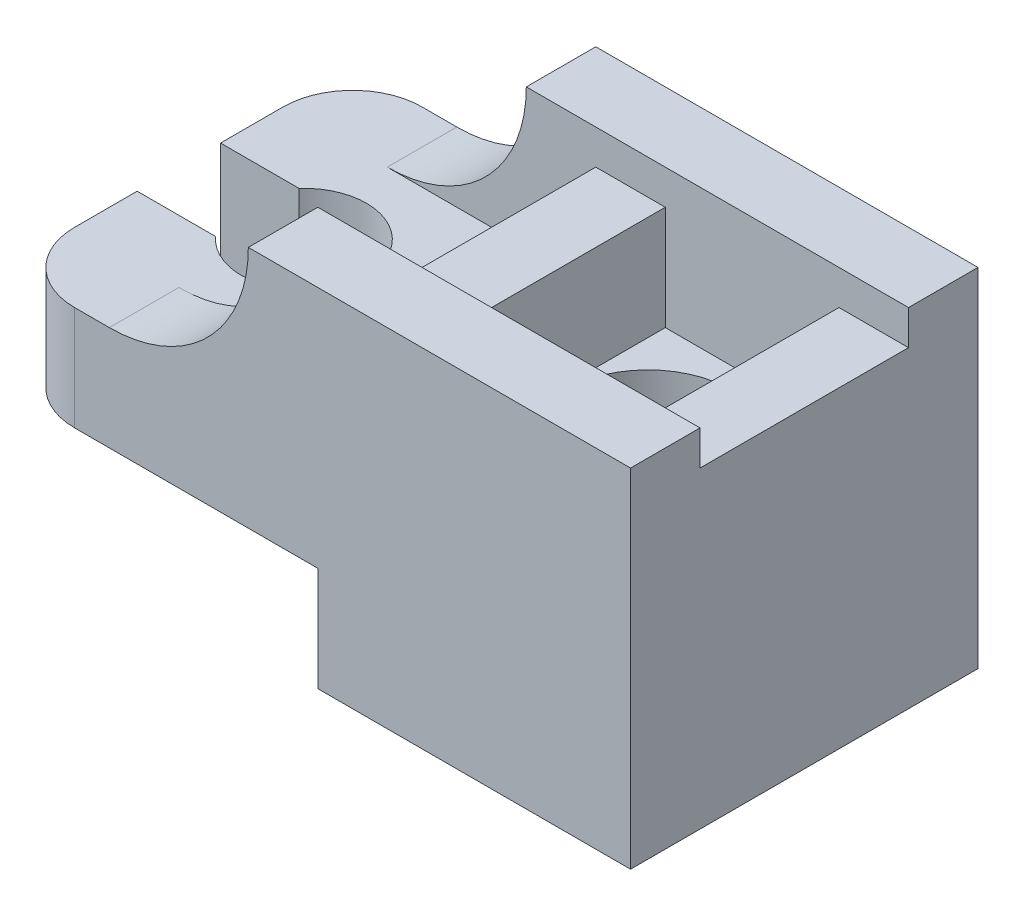
ISO-10303-21;
HEADER;
FILE_DESCRIPTION(('STEP AP214'),'2;1');
FILE_NAME('part.step','',(''),(''),'','','');
FILE_SCHEMA(('AUTOMOTIVE_DESIGN { 1 0 10303 214 1 1 1 1 }'));
ENDSEC;
DATA;
#1=APPLICATION_CONTEXT('core data for automotive mechanical design processes');
#2=APPLICATION_PROTOCOL_DEFINITION('international standard','automotive_design',2000,#1);
#3=PRODUCT_CONTEXT('',#1,'mechanical');
#4=PRODUCT('Part','Part','',(#3));
#5=PRODUCT_RELATED_PRODUCT_CATEGORY('part','',(#4));
#6=PRODUCT_DEFINITION_FORMATION('','',#4);
#7=PRODUCT_DEFINITION_CONTEXT('part definition',#1,'design');
#8=PRODUCT_DEFINITION('design','',#6,#7);
#9=PRODUCT_DEFINITION_SHAPE('','',#8);
#10=(LENGTH_UNIT() NAMED_UNIT(*) SI_UNIT(.MILLI.,.METRE.));
#11=(NAMED_UNIT(*) PLANE_ANGLE_UNIT() SI_UNIT($,.RADIAN.));
#12=(NAMED_UNIT(*) SI_UNIT($,.STERADIAN.) SOLID_ANGLE_UNIT());
#13=UNCERTAINTY_MEASURE_WITH_UNIT(LENGTH_MEASURE(1.E-05),#10,'distance_accuracy_value','');
#14=(GEOMETRIC_REPRESENTATION_CONTEXT(3) GLOBAL_UNCERTAINTY_ASSIGNED_CONTEXT((#13)) GLOBAL_UNIT_ASSIGNED_CONTEXT((#10,
#11,#12)) REPRESENTATION_CONTEXT('',''));
#15=CARTESIAN_POINT('',(0.,0.,0.));
#16=DIRECTION('',(0.,0.,1.));
#17=DIRECTION('',(1.,0.,0.));
#18=AXIS2_PLACEMENT_3D('',#15,#16,#17);
#19=CARTESIAN_POINT('',(90.,35.,-50.));
#20=DIRECTION('',(0.,1.,0.));
#21=DIRECTION('',(0.,0.,1.));
#22=AXIS2_PLACEMENT_3D('',#19,#20,#21);
#23=PLANE('',#22);
#24=DIRECTION('',(0.,0.,1.));
#25=VECTOR('',#24,1.);
#26=CARTESIAN_POINT('',(35.,35.,-50.));
#27=LINE('',#26,#25);
#28=CARTESIAN_POINT('',(35.,35.,-50.));
#29=VERTEX_POINT('',#28);
#30=CARTESIAN_POINT('',(35.,35.,-40.));
#31=VERTEX_POINT('',#30);
#32=EDGE_CURVE('E339',#29,#31,#27,.T.);
#33=ORIENTED_EDGE('',*,*,#32,.T.);
#34=DIRECTION('',(-1.,0.,0.));
#35=VECTOR('',#34,1.);
#36=CARTESIAN_POINT('',(95.,35.,-40.));
#37=LINE('',#36,#35);
#38=CARTESIAN_POINT('',(90.,35.,-40.));
#39=VERTEX_POINT('',#38);
#40=EDGE_CURVE('E258',#39,#31,#37,.T.);
#41=ORIENTED_EDGE('',*,*,#40,.F.);
#42=DIRECTION('',(0.,0.,1.));
#43=VECTOR('',#42,1.);
#44=CARTESIAN_POINT('',(90.,35.,-50.));
#45=LINE('',#44,#43);
#46=CARTESIAN_POINT('',(90.,35.,-50.));
#47=VERTEX_POINT('',#46);
#48=EDGE_CURVE('E344',#47,#39,#45,.T.);
#49=ORIENTED_EDGE('',*,*,#48,.F.);
#50=DIRECTION('',(-1.,0.,0.));
#51=VECTOR('',#50,1.);
#52=CARTESIAN_POINT('',(90.,35.,-50.));
#53=LINE('',#52,#51);
#54=EDGE_CURVE('E331',#47,#29,#53,.T.);
#55=ORIENTED_EDGE('',*,*,#54,.T.);
#56=EDGE_LOOP('',(#33,#41,#49,#55));
#57=FACE_BOUND('',#56,.T.);
#58=ADVANCED_FACE('F44',(#57),#23,.T.);
#59=CARTESIAN_POINT('',(90.,15.,-50.));
#60=DIRECTION('',(0.,1.,0.));
#61=DIRECTION('',(0.,0.,1.));
#62=AXIS2_PLACEMENT_3D('',#59,#60,#61);
#63=PLANE('',#62);
#64=CARTESIAN_POINT('',(67.5,15.,-25.));
#65=DIRECTION('',(0.,1.,0.));
#66=DIRECTION('',(0.,0.,1.));
#67=AXIS2_PLACEMENT_3D('',#64,#65,#66);
#68=CIRCLE('',#67,12.);
#69=CARTESIAN_POINT('',(67.5,15.,-13.));
#70=VERTEX_POINT('',#69);
#71=EDGE_CURVE('E802',#70,#70,#68,.T.);
#72=ORIENTED_EDGE('',*,*,#71,.F.);
#73=EDGE_LOOP('',(#72));
#74=FACE_BOUND('',#73,.T.);
#75=DIRECTION('',(0.,0.,-1.));
#76=VECTOR('',#75,1.);
#77=CARTESIAN_POINT('',(55.,15.,-40.));
#78=LINE('',#77,#76);
#79=CARTESIAN_POINT('',(55.,15.,-10.));
#80=VERTEX_POINT('',#79);
#81=CARTESIAN_POINT('',(55.,15.,-40.));
#82=VERTEX_POINT('',#81);
#83=EDGE_CURVE('E68',#80,#82,#78,.T.);
#84=ORIENTED_EDGE('',*,*,#83,.F.);
#85=DIRECTION('',(1.,0.,0.));
#86=VECTOR('',#85,1.);
#87=CARTESIAN_POINT('',(35.,15.,-10.));
#88=LINE('',#87,#86);
#89=CARTESIAN_POINT('',(80.,15.,-10.));
#90=VERTEX_POINT('',#89);
#91=EDGE_CURVE('E304',#80,#90,#88,.T.);
#92=ORIENTED_EDGE('',*,*,#91,.T.);
#93=DIRECTION('',(0.,0.,-1.));
#94=VECTOR('',#93,1.);
#95=CARTESIAN_POINT('',(80.,15.,-40.));
#96=LINE('',#95,#94);
#97=CARTESIAN_POINT('',(80.,15.,-40.));
#98=VERTEX_POINT('',#97);
#99=EDGE_CURVE('E251',#90,#98,#96,.T.);
#100=ORIENTED_EDGE('',*,*,#99,.T.);
#101=DIRECTION('',(-1.,0.,0.));
#102=VECTOR('',#101,1.);
#103=CARTESIAN_POINT('',(35.,15.,-40.));
#104=LINE('',#103,#102);
#105=EDGE_CURVE('E295',#98,#82,#104,.T.);
#106=ORIENTED_EDGE('',*,*,#105,.T.);
#107=EDGE_LOOP('',(#84,#92,#100,#106));
#108=FACE_BOUND('',#107,.T.);
#109=ADVANCED_FACE('F468',(#74,#108),#63,.T.);
#110=CARTESIAN_POINT('',(0.,15.,-50.));
#111=DIRECTION('',(-1.,0.,0.));
#112=DIRECTION('',(0.,0.,1.));
#113=AXIS2_PLACEMENT_3D('',#110,#111,#112);
#114=PLANE('',#113);
#115=DIRECTION('',(0.,1.,0.));
#116=VECTOR('',#115,1.);
#117=CARTESIAN_POINT('',(0.,0.,-31.));
#118=LINE('',#117,#116);
#119=CARTESIAN_POINT('',(0.,0.,-31.));
#120=VERTEX_POINT('',#119);
#121=CARTESIAN_POINT('',(0.,15.,-31.));
#122=VERTEX_POINT('',#121);
#123=EDGE_CURVE('E284',#120,#122,#118,.T.);
#124=ORIENTED_EDGE('',*,*,#123,.T.);
#125=DIRECTION('',(0.,0.,1.));
#126=VECTOR('',#125,1.);
#127=CARTESIAN_POINT('',(0.,15.,-50.));
#128=LINE('',#127,#126);
#129=CARTESIAN_POINT('',(0.,15.,-40.));
#130=VERTEX_POINT('',#129);
#131=EDGE_CURVE('E378',#130,#122,#128,.T.);
#132=ORIENTED_EDGE('',*,*,#131,.F.);
#133=DIRECTION('',(0.,1.,0.));
#134=VECTOR('',#133,1.);
#135=CARTESIAN_POINT('',(0.,-35.,-40.));
#136=LINE('',#135,#134);
#137=CARTESIAN_POINT('',(0.,0.,-40.));
#138=VERTEX_POINT('',#137);
#139=EDGE_CURVE('E316',#138,#130,#136,.T.);
#140=ORIENTED_EDGE('',*,*,#139,.F.);
#141=DIRECTION('',(0.,0.,1.));
#142=VECTOR('',#141,1.);
#143=CARTESIAN_POINT('',(0.,0.,-50.));
#144=LINE('',#143,#142);
#145=EDGE_CURVE('E384',#138,#120,#144,.T.);
#146=ORIENTED_EDGE('',*,*,#145,.T.);
#147=EDGE_LOOP('',(#124,#132,#140,#146));
#148=FACE_BOUND('',#147,.T.);
#149=ADVANCED_FACE('F450',(#148),#114,.T.);
#150=DIRECTION('',(0.,0.,1.));
#151=VECTOR('',#150,1.);
#152=CARTESIAN_POINT('',(45.,15.,-10.));
#153=LINE('',#152,#151);
#154=CARTESIAN_POINT('',(45.,15.,-40.));
#155=VERTEX_POINT('',#154);
#156=CARTESIAN_POINT('',(45.,15.,-10.));
#157=VERTEX_POINT('',#156);
#158=EDGE_CURVE('E227',#155,#157,#153,.T.);
#159=ORIENTED_EDGE('',*,*,#158,.F.);
#160=CARTESIAN_POINT('',(14.9999999999998,15.,-40.));
#161=VERTEX_POINT('',#160);
#162=EDGE_CURVE('E291',#155,#161,#104,.T.);
#163=ORIENTED_EDGE('',*,*,#162,.T.);
#164=DIRECTION('',(0.,0.,-1.));
#165=VECTOR('',#164,1.);
#166=CARTESIAN_POINT('',(14.9999999999998,15.,-40.));
#167=LINE('',#166,#165);
#168=CARTESIAN_POINT('',(14.9999999999998,15.,-50.));
#169=VERTEX_POINT('',#168);
#170=EDGE_CURVE('E298',#161,#169,#167,.T.);
#171=ORIENTED_EDGE('',*,*,#170,.T.);
#172=DIRECTION('',(-1.,0.,0.));
#173=VECTOR('',#172,1.);
#174=CARTESIAN_POINT('',(90.,15.,-50.));
#175=LINE('',#174,#173);
#176=CARTESIAN_POINT('',(10.,15.,-50.));
#177=VERTEX_POINT('',#176);
#178=EDGE_CURVE('E371',#169,#177,#175,.T.);
#179=ORIENTED_EDGE('',*,*,#178,.T.);
#180=CARTESIAN_POINT('',(10.,15.,-40.));
#181=DIRECTION('',(0.,1.,0.));
#182=DIRECTION('',(0.,0.,1.));
#183=AXIS2_PLACEMENT_3D('',#180,#181,#182);
#184=CIRCLE('',#183,10.);
#185=EDGE_CURVE('E317',#177,#130,#184,.T.);
#186=ORIENTED_EDGE('',*,*,#185,.T.);
#187=ORIENTED_EDGE('',*,*,#131,.T.);
#188=DIRECTION('',(-1.,0.,0.));
#189=VECTOR('',#188,1.);
#190=CARTESIAN_POINT('',(0.,15.,-31.));
#191=LINE('',#190,#189);
#192=CARTESIAN_POINT('',(11.2917960675006,15.,-31.));
#193=VERTEX_POINT('',#192);
#194=EDGE_CURVE('E266',#193,#122,#191,.T.);
#195=ORIENTED_EDGE('',*,*,#194,.F.);
#196=CARTESIAN_POINT('',(18.,15.,-25.));
#197=DIRECTION('',(0.,1.,0.));
#198=DIRECTION('',(0.,0.,1.));
#199=AXIS2_PLACEMENT_3D('',#196,#197,#198);
#200=CIRCLE('',#199,9.);
#201=CARTESIAN_POINT('',(11.2917960675006,15.,-19.));
#202=VERTEX_POINT('',#201);
#203=EDGE_CURVE('E280',#202,#193,#200,.T.);
#204=ORIENTED_EDGE('',*,*,#203,.F.);
#205=DIRECTION('',(1.,0.,0.));
#206=VECTOR('',#205,1.);
#207=CARTESIAN_POINT('',(11.2917960675006,15.,-19.));
#208=LINE('',#207,#206);
#209=CARTESIAN_POINT('',(0.,15.,-19.));
#210=VERTEX_POINT('',#209);
#211=EDGE_CURVE('E261',#210,#202,#208,.T.);
#212=ORIENTED_EDGE('',*,*,#211,.F.);
#213=CARTESIAN_POINT('',(0.,15.,-10.));
#214=VERTEX_POINT('',#213);
#215=EDGE_CURVE('E385',#210,#214,#128,.T.);
#216=ORIENTED_EDGE('',*,*,#215,.T.);
#217=CARTESIAN_POINT('',(10.,15.,-10.));
#218=DIRECTION('',(0.,1.,0.));
#219=DIRECTION('',(0.,0.,1.));
#220=AXIS2_PLACEMENT_3D('',#217,#218,#219);
#221=CIRCLE('',#220,10.);
#222=CARTESIAN_POINT('',(10.,15.,0.));
#223=VERTEX_POINT('',#222);
#224=EDGE_CURVE('E313',#214,#223,#221,.T.);
#225=ORIENTED_EDGE('',*,*,#224,.T.);
#226=DIRECTION('',(-1.,0.,0.));
#227=VECTOR('',#226,1.);
#228=CARTESIAN_POINT('',(90.,15.,0.));
#229=LINE('',#228,#227);
#230=CARTESIAN_POINT('',(15.,15.,0.));
#231=VERTEX_POINT('',#230);
#232=EDGE_CURVE('E367',#231,#223,#229,.T.);
#233=ORIENTED_EDGE('',*,*,#232,.F.);
#234=DIRECTION('',(0.,0.,1.));
#235=VECTOR('',#234,1.);
#236=CARTESIAN_POINT('',(15.,15.,-10.));
#237=LINE('',#236,#235);
#238=CARTESIAN_POINT('',(15.,15.,-10.));
#239=VERTEX_POINT('',#238);
#240=EDGE_CURVE('E308',#239,#231,#237,.T.);
#241=ORIENTED_EDGE('',*,*,#240,.F.);
#242=EDGE_CURVE('E306',#239,#157,#88,.T.);
#243=ORIENTED_EDGE('',*,*,#242,.T.);
#244=EDGE_LOOP('',(#159,#163,#171,#179,#186,#187,#195,#204,#212,#216,#225,#233,#241,#243));
#245=FACE_BOUND('',#244,.T.);
#246=ADVANCED_FACE('F398',(#245),#63,.T.);
#247=CARTESIAN_POINT('',(0.,0.,-50.));
#248=DIRECTION('',(0.,-1.,0.));
#249=DIRECTION('',(0.,0.,-1.));
#250=AXIS2_PLACEMENT_3D('',#247,#248,#249);
#251=PLANE('',#250);
#252=DIRECTION('',(-1.,0.,0.));
#253=VECTOR('',#252,1.);
#254=CARTESIAN_POINT('',(0.,0.,-31.));
#255=LINE('',#254,#253);
#256=CARTESIAN_POINT('',(11.2917960675006,0.,-31.));
#257=VERTEX_POINT('',#256);
#258=EDGE_CURVE('E272',#257,#120,#255,.T.);
#259=ORIENTED_EDGE('',*,*,#258,.T.);
#260=ORIENTED_EDGE('',*,*,#145,.F.);
#261=CARTESIAN_POINT('',(10.,0.,-40.));
#262=DIRECTION('',(0.,-1.,0.));
#263=DIRECTION('',(0.,0.,-1.));
#264=AXIS2_PLACEMENT_3D('',#261,#262,#263);
#265=CIRCLE('',#264,10.);
#266=CARTESIAN_POINT('',(10.,0.,-50.));
#267=VERTEX_POINT('',#266);
#268=EDGE_CURVE('E328',#138,#267,#265,.T.);
#269=ORIENTED_EDGE('',*,*,#268,.T.);
#270=DIRECTION('',(1.,0.,0.));
#271=VECTOR('',#270,1.);
#272=CARTESIAN_POINT('',(0.,0.,-50.));
#273=LINE('',#272,#271);
#274=CARTESIAN_POINT('',(45.,0.,-50.));
#275=VERTEX_POINT('',#274);
#276=EDGE_CURVE('E366',#267,#275,#273,.T.);
#277=ORIENTED_EDGE('',*,*,#276,.T.);
#278=DIRECTION('',(0.,0.,1.));
#279=VECTOR('',#278,1.);
#280=CARTESIAN_POINT('',(45.,0.,-50.));
#281=LINE('',#280,#279);
#282=CARTESIAN_POINT('',(45.,0.,0.));
#283=VERTEX_POINT('',#282);
#284=EDGE_CURVE('E351',#275,#283,#281,.T.);
#285=ORIENTED_EDGE('',*,*,#284,.T.);
#286=DIRECTION('',(1.,0.,0.));
#287=VECTOR('',#286,1.);
#288=CARTESIAN_POINT('',(0.,0.,0.));
#289=LINE('',#288,#287);
#290=CARTESIAN_POINT('',(10.,0.,0.));
#291=VERTEX_POINT('',#290);
#292=EDGE_CURVE('E363',#291,#283,#289,.T.);
#293=ORIENTED_EDGE('',*,*,#292,.F.);
#294=CARTESIAN_POINT('',(10.,0.,-10.));
#295=DIRECTION('',(0.,-1.,0.));
#296=DIRECTION('',(0.,0.,-1.));
#297=AXIS2_PLACEMENT_3D('',#294,#295,#296);
#298=CIRCLE('',#297,10.);
#299=CARTESIAN_POINT('',(0.,0.,-10.));
#300=VERTEX_POINT('',#299);
#301=EDGE_CURVE('E325',#291,#300,#298,.T.);
#302=ORIENTED_EDGE('',*,*,#301,.T.);
#303=CARTESIAN_POINT('',(0.,0.,-19.));
#304=VERTEX_POINT('',#303);
#305=EDGE_CURVE('E373',#304,#300,#144,.T.);
#306=ORIENTED_EDGE('',*,*,#305,.F.);
#307=DIRECTION('',(1.,0.,0.));
#308=VECTOR('',#307,1.);
#309=CARTESIAN_POINT('',(11.2917960675006,0.,-19.));
#310=LINE('',#309,#308);
#311=CARTESIAN_POINT('',(11.2917960675006,0.,-19.));
#312=VERTEX_POINT('',#311);
#313=EDGE_CURVE('E263',#304,#312,#310,.T.);
#314=ORIENTED_EDGE('',*,*,#313,.T.);
#315=CARTESIAN_POINT('',(18.,0.,-25.));
#316=DIRECTION('',(0.,1.,0.));
#317=DIRECTION('',(0.,0.,1.));
#318=AXIS2_PLACEMENT_3D('',#315,#316,#317);
#319=CIRCLE('',#318,9.);
#320=EDGE_CURVE('E270',#312,#257,#319,.T.);
#321=ORIENTED_EDGE('',*,*,#320,.T.);
#322=EDGE_LOOP('',(#259,#260,#269,#277,#285,#293,#302,#306,#314,#321));
#323=FACE_BOUND('',#322,.T.);
#324=ADVANCED_FACE('F403',(#323),#251,.T.);
#325=DIRECTION('',(0.,1.,0.));
#326=VECTOR('',#325,1.);
#327=CARTESIAN_POINT('',(0.,0.,-19.));
#328=LINE('',#327,#326);
#329=EDGE_CURVE('E274',#304,#210,#328,.T.);
#330=ORIENTED_EDGE('',*,*,#329,.F.);
#331=ORIENTED_EDGE('',*,*,#305,.T.);
#332=DIRECTION('',(0.,1.,0.));
#333=VECTOR('',#332,1.);
#334=CARTESIAN_POINT('',(0.,-35.,-10.));
#335=LINE('',#334,#333);
#336=EDGE_CURVE('E318',#300,#214,#335,.T.);
#337=ORIENTED_EDGE('',*,*,#336,.T.);
#338=ORIENTED_EDGE('',*,*,#215,.F.);
#339=EDGE_LOOP('',(#330,#331,#337,#338));
#340=FACE_BOUND('',#339,.T.);
#341=ADVANCED_FACE('F50',(#340),#114,.T.);
#342=CARTESIAN_POINT('',(90.,0.,-50.));
#343=DIRECTION('',(1.,0.,0.));
#344=DIRECTION('',(0.,0.,-1.));
#345=AXIS2_PLACEMENT_3D('',#342,#343,#344);
#346=PLANE('',#345);
#347=DIRECTION('',(0.,1.,0.));
#348=VECTOR('',#347,1.);
#349=CARTESIAN_POINT('',(90.,30.,-40.));
#350=LINE('',#349,#348);
#351=CARTESIAN_POINT('',(90.,30.,-40.));
#352=VERTEX_POINT('',#351);
#353=EDGE_CURVE('E246',#352,#39,#350,.T.);
#354=ORIENTED_EDGE('',*,*,#353,.F.);
#355=DIRECTION('',(0.,0.,-1.));
#356=VECTOR('',#355,1.);
#357=CARTESIAN_POINT('',(90.,30.,-40.));
#358=LINE('',#357,#356);
#359=CARTESIAN_POINT('',(90.,30.,-9.99999999999999));
#360=VERTEX_POINT('',#359);
#361=EDGE_CURVE('E241',#360,#352,#358,.T.);
#362=ORIENTED_EDGE('',*,*,#361,.F.);
#363=DIRECTION('',(0.,1.,0.));
#364=VECTOR('',#363,1.);
#365=CARTESIAN_POINT('',(90.,30.,-9.99999999999999));
#366=LINE('',#365,#364);
#367=CARTESIAN_POINT('',(90.,35.,-9.99999999999999));
#368=VERTEX_POINT('',#367);
#369=EDGE_CURVE('E244',#360,#368,#366,.T.);
#370=ORIENTED_EDGE('',*,*,#369,.T.);
#371=CARTESIAN_POINT('',(90.,35.,0.));
#372=VERTEX_POINT('',#371);
#373=EDGE_CURVE('E337',#368,#372,#45,.T.);
#374=ORIENTED_EDGE('',*,*,#373,.T.);
#375=DIRECTION('',(0.,1.,0.));
#376=VECTOR('',#375,1.);
#377=CARTESIAN_POINT('',(90.,0.,0.));
#378=LINE('',#377,#376);
#379=CARTESIAN_POINT('',(90.,-15.,0.));
#380=VERTEX_POINT('',#379);
#381=EDGE_CURVE('E374',#380,#372,#378,.T.);
#382=ORIENTED_EDGE('',*,*,#381,.F.);
#383=DIRECTION('',(0.,0.,1.));
#384=VECTOR('',#383,1.);
#385=CARTESIAN_POINT('',(90.,-15.,-50.));
#386=LINE('',#385,#384);
#387=CARTESIAN_POINT('',(90.,-15.,-50.));
#388=VERTEX_POINT('',#387);
#389=EDGE_CURVE('E356',#388,#380,#386,.T.);
#390=ORIENTED_EDGE('',*,*,#389,.F.);
#391=DIRECTION('',(0.,1.,0.));
#392=VECTOR('',#391,1.);
#393=CARTESIAN_POINT('',(90.,0.,-50.));
#394=LINE('',#393,#392);
#395=EDGE_CURVE('E368',#388,#47,#394,.T.);
#396=ORIENTED_EDGE('',*,*,#395,.T.);
#397=ORIENTED_EDGE('',*,*,#48,.T.);
#398=EDGE_LOOP('',(#354,#362,#370,#374,#382,#390,#396,#397));
#399=FACE_BOUND('',#398,.T.);
#400=ADVANCED_FACE('F494',(#399),#346,.T.);
#401=CARTESIAN_POINT('',(0.,0.,-50.));
#402=DIRECTION('',(0.,0.,1.));
#403=DIRECTION('',(1.,0.,0.));
#404=AXIS2_PLACEMENT_3D('',#401,#402,#403);
#405=PLANE('',#404);
#406=ORIENTED_EDGE('',*,*,#178,.F.);
#407=CARTESIAN_POINT('',(15.,35.,-50.));
#408=DIRECTION('',(0.,0.,1.));
#409=DIRECTION('',(-1.,0.,0.));
#410=AXIS2_PLACEMENT_3D('',#407,#408,#409);
#411=CIRCLE('',#410,20.);
#412=EDGE_CURVE('E283',#169,#29,#411,.T.);
#413=ORIENTED_EDGE('',*,*,#412,.T.);
#414=ORIENTED_EDGE('',*,*,#54,.F.);
#415=ORIENTED_EDGE('',*,*,#395,.F.);
#416=DIRECTION('',(1.,0.,0.));
#417=VECTOR('',#416,1.);
#418=CARTESIAN_POINT('',(90.,-15.,-50.));
#419=LINE('',#418,#417);
#420=CARTESIAN_POINT('',(45.,-15.,-50.));
#421=VERTEX_POINT('',#420);
#422=EDGE_CURVE('E348',#421,#388,#419,.T.);
#423=ORIENTED_EDGE('',*,*,#422,.F.);
#424=DIRECTION('',(0.,-1.,0.));
#425=VECTOR('',#424,1.);
#426=CARTESIAN_POINT('',(45.,-15.,-50.));
#427=LINE('',#426,#425);
#428=EDGE_CURVE('E349',#275,#421,#427,.T.);
#429=ORIENTED_EDGE('',*,*,#428,.F.);
#430=ORIENTED_EDGE('',*,*,#276,.F.);
#431=DIRECTION('',(0.,1.,0.));
#432=VECTOR('',#431,1.);
#433=CARTESIAN_POINT('',(10.,-35.,-50.));
#434=LINE('',#433,#432);
#435=EDGE_CURVE('E11',#267,#177,#434,.T.);
#436=ORIENTED_EDGE('',*,*,#435,.T.);
#437=EDGE_LOOP('',(#406,#413,#414,#415,#423,#429,#430,#436));
#438=FACE_BOUND('',#437,.T.);
#439=ADVANCED_FACE('F438',(#438),#405,.F.);
#440=CARTESIAN_POINT('',(0.,0.,0.));
#441=DIRECTION('',(0.,0.,1.));
#442=DIRECTION('',(1.,0.,0.));
#443=AXIS2_PLACEMENT_3D('',#440,#441,#442);
#444=PLANE('',#443);
#445=CARTESIAN_POINT('',(15.,35.,0.));
#446=DIRECTION('',(0.,0.,-1.));
#447=DIRECTION('',(1.,0.,0.));
#448=AXIS2_PLACEMENT_3D('',#445,#446,#447);
#449=CIRCLE('',#448,20.);
#450=CARTESIAN_POINT('',(35.,35.,0.));
#451=VERTEX_POINT('',#450);
#452=EDGE_CURVE('E301',#451,#231,#449,.T.);
#453=ORIENTED_EDGE('',*,*,#452,.T.);
#454=ORIENTED_EDGE('',*,*,#232,.T.);
#455=DIRECTION('',(0.,1.,0.));
#456=VECTOR('',#455,1.);
#457=CARTESIAN_POINT('',(10.,-35.,0.));
#458=LINE('',#457,#456);
#459=EDGE_CURVE('E53',#291,#223,#458,.T.);
#460=ORIENTED_EDGE('',*,*,#459,.F.);
#461=ORIENTED_EDGE('',*,*,#292,.T.);
#462=DIRECTION('',(0.,-1.,0.));
#463=VECTOR('',#462,1.);
#464=CARTESIAN_POINT('',(45.,-15.,0.));
#465=LINE('',#464,#463);
#466=CARTESIAN_POINT('',(45.,-15.,0.));
#467=VERTEX_POINT('',#466);
#468=EDGE_CURVE('E345',#283,#467,#465,.T.);
#469=ORIENTED_EDGE('',*,*,#468,.T.);
#470=DIRECTION('',(1.,0.,0.));
#471=VECTOR('',#470,1.);
#472=CARTESIAN_POINT('',(90.,-15.,0.));
#473=LINE('',#472,#471);
#474=EDGE_CURVE('E347',#467,#380,#473,.T.);
#475=ORIENTED_EDGE('',*,*,#474,.T.);
#476=ORIENTED_EDGE('',*,*,#381,.T.);
#477=DIRECTION('',(-1.,0.,0.));
#478=VECTOR('',#477,1.);
#479=CARTESIAN_POINT('',(90.,35.,0.));
#480=LINE('',#479,#478);
#481=EDGE_CURVE('E335',#372,#451,#480,.T.);
#482=ORIENTED_EDGE('',*,*,#481,.T.);
#483=EDGE_LOOP('',(#453,#454,#460,#461,#469,#475,#476,#482));
#484=FACE_BOUND('',#483,.T.);
#485=ADVANCED_FACE('F409',(#484),#444,.T.);
#486=CARTESIAN_POINT('',(90.,-15.,-50.));
#487=DIRECTION('',(0.,-1.,0.));
#488=DIRECTION('',(0.,0.,-1.));
#489=AXIS2_PLACEMENT_3D('',#486,#487,#488);
#490=PLANE('',#489);
#491=CARTESIAN_POINT('',(67.5,-15.,-25.));
#492=DIRECTION('',(0.,-1.,0.));
#493=DIRECTION('',(0.,0.,-1.));
#494=AXIS2_PLACEMENT_3D('',#491,#492,#493);
#495=CIRCLE('',#494,12.);
#496=CARTESIAN_POINT('',(67.5,-15.,-37.));
#497=VERTEX_POINT('',#496);
#498=EDGE_CURVE('E47',#497,#497,#495,.T.);
#499=ORIENTED_EDGE('',*,*,#498,.F.);
#500=EDGE_LOOP('',(#499));
#501=FACE_BOUND('',#500,.T.);
#502=ORIENTED_EDGE('',*,*,#474,.F.);
#503=DIRECTION('',(0.,0.,1.));
#504=VECTOR('',#503,1.);
#505=CARTESIAN_POINT('',(45.,-15.,-50.));
#506=LINE('',#505,#504);
#507=EDGE_CURVE('E365',#421,#467,#506,.T.);
#508=ORIENTED_EDGE('',*,*,#507,.F.);
#509=ORIENTED_EDGE('',*,*,#422,.T.);
#510=ORIENTED_EDGE('',*,*,#389,.T.);
#511=EDGE_LOOP('',(#502,#508,#509,#510));
#512=FACE_BOUND('',#511,.T.);
#513=ADVANCED_FACE('F412',(#501,#512),#490,.T.);
#514=CARTESIAN_POINT('',(45.,-15.,-50.));
#515=DIRECTION('',(-1.,0.,0.));
#516=DIRECTION('',(0.,-1.,0.));
#517=AXIS2_PLACEMENT_3D('',#514,#515,#516);
#518=PLANE('',#517);
#519=ORIENTED_EDGE('',*,*,#468,.F.);
#520=ORIENTED_EDGE('',*,*,#284,.F.);
#521=ORIENTED_EDGE('',*,*,#428,.T.);
#522=ORIENTED_EDGE('',*,*,#507,.T.);
#523=EDGE_LOOP('',(#519,#520,#521,#522));
#524=FACE_BOUND('',#523,.T.);
#525=ADVANCED_FACE('F408',(#524),#518,.T.);
#526=DIRECTION('',(-1.,0.,0.));
#527=VECTOR('',#526,1.);
#528=CARTESIAN_POINT('',(95.,35.,-10.));
#529=LINE('',#528,#527);
#530=CARTESIAN_POINT('',(35.,35.,-10.));
#531=VERTEX_POINT('',#530);
#532=EDGE_CURVE('E256',#368,#531,#529,.T.);
#533=ORIENTED_EDGE('',*,*,#532,.T.);
#534=DIRECTION('',(0.,0.,1.));
#535=VECTOR('',#534,1.);
#536=CARTESIAN_POINT('',(35.,35.,-10.));
#537=LINE('',#536,#535);
#538=EDGE_CURVE('E311',#531,#451,#537,.T.);
#539=ORIENTED_EDGE('',*,*,#538,.T.);
#540=ORIENTED_EDGE('',*,*,#481,.F.);
#541=ORIENTED_EDGE('',*,*,#373,.F.);
#542=EDGE_LOOP('',(#533,#539,#540,#541));
#543=FACE_BOUND('',#542,.T.);
#544=ADVANCED_FACE('F423',(#543),#23,.T.);
#545=CARTESIAN_POINT('',(10.,-35.,-10.));
#546=DIRECTION('',(0.,1.,0.));
#547=DIRECTION('',(0.,0.,1.));
#548=AXIS2_PLACEMENT_3D('',#545,#546,#547);
#549=CYLINDRICAL_SURFACE('',#548,10.);
#550=ORIENTED_EDGE('',*,*,#459,.T.);
#551=ORIENTED_EDGE('',*,*,#224,.F.);
#552=ORIENTED_EDGE('',*,*,#336,.F.);
#553=ORIENTED_EDGE('',*,*,#301,.F.);
#554=EDGE_LOOP('',(#550,#551,#552,#553));
#555=FACE_BOUND('',#554,.T.);
#556=ADVANCED_FACE('F388',(#555),#549,.T.);
#557=CARTESIAN_POINT('',(10.,-35.,-40.));
#558=DIRECTION('',(0.,1.,0.));
#559=DIRECTION('',(0.,0.,1.));
#560=AXIS2_PLACEMENT_3D('',#557,#558,#559);
#561=CYLINDRICAL_SURFACE('',#560,10.);
#562=ORIENTED_EDGE('',*,*,#139,.T.);
#563=ORIENTED_EDGE('',*,*,#185,.F.);
#564=ORIENTED_EDGE('',*,*,#435,.F.);
#565=ORIENTED_EDGE('',*,*,#268,.F.);
#566=EDGE_LOOP('',(#562,#563,#564,#565));
#567=FACE_BOUND('',#566,.T.);
#568=ADVANCED_FACE('F445',(#567),#561,.T.);
#569=CARTESIAN_POINT('',(15.,35.,-10.));
#570=DIRECTION('',(0.,0.,1.));
#571=DIRECTION('',(1.,0.,0.));
#572=AXIS2_PLACEMENT_3D('',#569,#570,#571);
#573=CYLINDRICAL_SURFACE('',#572,20.);
#574=ORIENTED_EDGE('',*,*,#452,.F.);
#575=ORIENTED_EDGE('',*,*,#538,.F.);
#576=CARTESIAN_POINT('',(15.,35.,-10.));
#577=DIRECTION('',(0.,0.,-1.));
#578=DIRECTION('',(1.,0.,0.));
#579=AXIS2_PLACEMENT_3D('',#576,#577,#578);
#580=CIRCLE('',#579,20.);
#581=EDGE_CURVE('E305',#531,#239,#580,.T.);
#582=ORIENTED_EDGE('',*,*,#581,.T.);
#583=ORIENTED_EDGE('',*,*,#240,.T.);
#584=EDGE_LOOP('',(#574,#575,#582,#583));
#585=FACE_BOUND('',#584,.T.);
#586=ADVANCED_FACE('F425',(#585),#573,.F.);
#587=CARTESIAN_POINT('',(15.,35.,-10.));
#588=DIRECTION('',(0.,0.,1.));
#589=DIRECTION('',(1.,0.,0.));
#590=AXIS2_PLACEMENT_3D('',#587,#588,#589);
#591=PLANE('',#590);
#592=ORIENTED_EDGE('',*,*,#581,.F.);
#593=ORIENTED_EDGE('',*,*,#532,.F.);
#594=ORIENTED_EDGE('',*,*,#369,.F.);
#595=DIRECTION('',(1.,0.,0.));
#596=VECTOR('',#595,1.);
#597=CARTESIAN_POINT('',(90.,30.,-9.99999999999999));
#598=LINE('',#597,#596);
#599=CARTESIAN_POINT('',(80.,30.,-10.));
#600=VERTEX_POINT('',#599);
#601=EDGE_CURVE('E238',#600,#360,#598,.T.);
#602=ORIENTED_EDGE('',*,*,#601,.F.);
#603=DIRECTION('',(0.,-1.,0.));
#604=VECTOR('',#603,1.);
#605=CARTESIAN_POINT('',(80.,15.,-10.));
#606=LINE('',#605,#604);
#607=EDGE_CURVE('E248',#600,#90,#606,.T.);
#608=ORIENTED_EDGE('',*,*,#607,.T.);
#609=ORIENTED_EDGE('',*,*,#91,.F.);
#610=DIRECTION('',(0.,1.,0.));
#611=VECTOR('',#610,1.);
#612=CARTESIAN_POINT('',(55.,15.,-10.));
#613=LINE('',#612,#611);
#614=CARTESIAN_POINT('',(55.,30.,-10.));
#615=VERTEX_POINT('',#614);
#616=EDGE_CURVE('E213',#80,#615,#613,.T.);
#617=ORIENTED_EDGE('',*,*,#616,.T.);
#618=DIRECTION('',(1.,0.,0.));
#619=VECTOR('',#618,1.);
#620=CARTESIAN_POINT('',(55.,30.,-10.));
#621=LINE('',#620,#619);
#622=CARTESIAN_POINT('',(45.,30.,-10.));
#623=VERTEX_POINT('',#622);
#624=EDGE_CURVE('E206',#623,#615,#621,.T.);
#625=ORIENTED_EDGE('',*,*,#624,.F.);
#626=DIRECTION('',(0.,1.,0.));
#627=VECTOR('',#626,1.);
#628=CARTESIAN_POINT('',(45.,15.,-10.));
#629=LINE('',#628,#627);
#630=EDGE_CURVE('E215',#157,#623,#629,.T.);
#631=ORIENTED_EDGE('',*,*,#630,.F.);
#632=ORIENTED_EDGE('',*,*,#242,.F.);
#633=EDGE_LOOP('',(#592,#593,#594,#602,#608,#609,#617,#625,#631,#632));
#634=FACE_BOUND('',#633,.T.);
#635=ADVANCED_FACE('F208',(#634),#591,.F.);
#636=CARTESIAN_POINT('',(15.,35.,-40.));
#637=DIRECTION('',(0.,0.,-1.));
#638=DIRECTION('',(-1.,0.,0.));
#639=AXIS2_PLACEMENT_3D('',#636,#637,#638);
#640=CYLINDRICAL_SURFACE('',#639,20.);
#641=ORIENTED_EDGE('',*,*,#412,.F.);
#642=ORIENTED_EDGE('',*,*,#170,.F.);
#643=CARTESIAN_POINT('',(15.,35.,-40.));
#644=DIRECTION('',(0.,0.,1.));
#645=DIRECTION('',(-1.,0.,0.));
#646=AXIS2_PLACEMENT_3D('',#643,#644,#645);
#647=CIRCLE('',#646,20.);
#648=EDGE_CURVE('E289',#161,#31,#647,.T.);
#649=ORIENTED_EDGE('',*,*,#648,.T.);
#650=ORIENTED_EDGE('',*,*,#32,.F.);
#651=EDGE_LOOP('',(#641,#642,#649,#650));
#652=FACE_BOUND('',#651,.T.);
#653=ADVANCED_FACE('F435',(#652),#640,.F.);
#654=CARTESIAN_POINT('',(15.,35.,-40.));
#655=DIRECTION('',(0.,0.,-1.));
#656=DIRECTION('',(-1.,0.,0.));
#657=AXIS2_PLACEMENT_3D('',#654,#655,#656);
#658=PLANE('',#657);
#659=ORIENTED_EDGE('',*,*,#162,.F.);
#660=DIRECTION('',(0.,1.,0.));
#661=VECTOR('',#660,1.);
#662=CARTESIAN_POINT('',(45.,15.,-40.));
#663=LINE('',#662,#661);
#664=CARTESIAN_POINT('',(45.,30.,-40.));
#665=VERTEX_POINT('',#664);
#666=EDGE_CURVE('E226',#155,#665,#663,.T.);
#667=ORIENTED_EDGE('',*,*,#666,.T.);
#668=DIRECTION('',(-1.,0.,0.));
#669=VECTOR('',#668,1.);
#670=CARTESIAN_POINT('',(45.,30.,-40.));
#671=LINE('',#670,#669);
#672=CARTESIAN_POINT('',(55.,30.,-40.));
#673=VERTEX_POINT('',#672);
#674=EDGE_CURVE('E62',#673,#665,#671,.T.);
#675=ORIENTED_EDGE('',*,*,#674,.F.);
#676=DIRECTION('',(0.,1.,0.));
#677=VECTOR('',#676,1.);
#678=CARTESIAN_POINT('',(55.,15.,-40.));
#679=LINE('',#678,#677);
#680=EDGE_CURVE('E229',#82,#673,#679,.T.);
#681=ORIENTED_EDGE('',*,*,#680,.F.);
#682=ORIENTED_EDGE('',*,*,#105,.F.);
#683=DIRECTION('',(0.,1.,0.));
#684=VECTOR('',#683,1.);
#685=CARTESIAN_POINT('',(80.,35.,-40.));
#686=LINE('',#685,#684);
#687=CARTESIAN_POINT('',(80.,30.,-40.));
#688=VERTEX_POINT('',#687);
#689=EDGE_CURVE('E257',#98,#688,#686,.T.);
#690=ORIENTED_EDGE('',*,*,#689,.T.);
#691=DIRECTION('',(-1.,0.,0.));
#692=VECTOR('',#691,1.);
#693=CARTESIAN_POINT('',(80.,30.,-40.));
#694=LINE('',#693,#692);
#695=EDGE_CURVE('E243',#352,#688,#694,.T.);
#696=ORIENTED_EDGE('',*,*,#695,.F.);
#697=ORIENTED_EDGE('',*,*,#353,.T.);
#698=ORIENTED_EDGE('',*,*,#40,.T.);
#699=ORIENTED_EDGE('',*,*,#648,.F.);
#700=EDGE_LOOP('',(#659,#667,#675,#681,#682,#690,#696,#697,#698,#699));
#701=FACE_BOUND('',#700,.T.);
#702=ADVANCED_FACE('F427',(#701),#658,.F.);
#703=CARTESIAN_POINT('',(0.,0.,-31.));
#704=DIRECTION('',(0.,0.,-1.));
#705=DIRECTION('',(-1.,0.,0.));
#706=AXIS2_PLACEMENT_3D('',#703,#704,#705);
#707=PLANE('',#706);
#708=ORIENTED_EDGE('',*,*,#194,.T.);
#709=ORIENTED_EDGE('',*,*,#123,.F.);
#710=ORIENTED_EDGE('',*,*,#258,.F.);
#711=DIRECTION('',(0.,1.,0.));
#712=VECTOR('',#711,1.);
#713=CARTESIAN_POINT('',(11.2917960675006,0.,-31.));
#714=LINE('',#713,#712);
#715=EDGE_CURVE('E282',#257,#193,#714,.T.);
#716=ORIENTED_EDGE('',*,*,#715,.T.);
#717=EDGE_LOOP('',(#708,#709,#710,#716));
#718=FACE_BOUND('',#717,.T.);
#719=ADVANCED_FACE('F448',(#718),#707,.F.);
#720=CARTESIAN_POINT('',(18.,0.,-25.));
#721=DIRECTION('',(0.,1.,0.));
#722=DIRECTION('',(0.,0.,1.));
#723=AXIS2_PLACEMENT_3D('',#720,#721,#722);
#724=CYLINDRICAL_SURFACE('',#723,9.);
#725=ORIENTED_EDGE('',*,*,#203,.T.);
#726=ORIENTED_EDGE('',*,*,#715,.F.);
#727=ORIENTED_EDGE('',*,*,#320,.F.);
#728=DIRECTION('',(0.,1.,0.));
#729=VECTOR('',#728,1.);
#730=CARTESIAN_POINT('',(11.2917960675006,0.,-19.));
#731=LINE('',#730,#729);
#732=EDGE_CURVE('E290',#312,#202,#731,.T.);
#733=ORIENTED_EDGE('',*,*,#732,.T.);
#734=EDGE_LOOP('',(#725,#726,#727,#733));
#735=FACE_BOUND('',#734,.T.);
#736=ADVANCED_FACE('F451',(#735),#724,.F.);
#737=CARTESIAN_POINT('',(11.2917960675006,0.,-19.));
#738=DIRECTION('',(0.,0.,1.));
#739=DIRECTION('',(1.,0.,0.));
#740=AXIS2_PLACEMENT_3D('',#737,#738,#739);
#741=PLANE('',#740);
#742=ORIENTED_EDGE('',*,*,#211,.T.);
#743=ORIENTED_EDGE('',*,*,#732,.F.);
#744=ORIENTED_EDGE('',*,*,#313,.F.);
#745=ORIENTED_EDGE('',*,*,#329,.T.);
#746=EDGE_LOOP('',(#742,#743,#744,#745));
#747=FACE_BOUND('',#746,.T.);
#748=ADVANCED_FACE('F459',(#747),#741,.F.);
#749=CARTESIAN_POINT('',(80.,0.,0.));
#750=DIRECTION('',(-1.,0.,0.));
#751=DIRECTION('',(0.,0.,1.));
#752=AXIS2_PLACEMENT_3D('',#749,#750,#751);
#753=PLANE('',#752);
#754=DIRECTION('',(0.,0.,1.));
#755=VECTOR('',#754,1.);
#756=CARTESIAN_POINT('',(80.,30.,-10.));
#757=LINE('',#756,#755);
#758=EDGE_CURVE('E232',#688,#600,#757,.T.);
#759=ORIENTED_EDGE('',*,*,#758,.F.);
#760=ORIENTED_EDGE('',*,*,#689,.F.);
#761=ORIENTED_EDGE('',*,*,#99,.F.);
#762=ORIENTED_EDGE('',*,*,#607,.F.);
#763=EDGE_LOOP('',(#759,#760,#761,#762));
#764=FACE_BOUND('',#763,.T.);
#765=ADVANCED_FACE('F460',(#764),#753,.T.);
#766=CARTESIAN_POINT('',(0.,30.,0.));
#767=DIRECTION('',(0.,-1.,0.));
#768=DIRECTION('',(0.,0.,-1.));
#769=AXIS2_PLACEMENT_3D('',#766,#767,#768);
#770=PLANE('',#769);
#771=ORIENTED_EDGE('',*,*,#758,.T.);
#772=ORIENTED_EDGE('',*,*,#601,.T.);
#773=ORIENTED_EDGE('',*,*,#361,.T.);
#774=ORIENTED_EDGE('',*,*,#695,.T.);
#775=EDGE_LOOP('',(#771,#772,#773,#774));
#776=FACE_BOUND('',#775,.T.);
#777=ADVANCED_FACE('F462',(#776),#770,.F.);
#778=CARTESIAN_POINT('',(55.,15.,-40.));
#779=DIRECTION('',(1.,0.,0.));
#780=DIRECTION('',(0.,0.,-1.));
#781=AXIS2_PLACEMENT_3D('',#778,#779,#780);
#782=PLANE('',#781);
#783=DIRECTION('',(0.,0.,-1.));
#784=VECTOR('',#783,1.);
#785=CARTESIAN_POINT('',(55.,30.,-40.));
#786=LINE('',#785,#784);
#787=EDGE_CURVE('E216',#615,#673,#786,.T.);
#788=ORIENTED_EDGE('',*,*,#787,.F.);
#789=ORIENTED_EDGE('',*,*,#616,.F.);
#790=ORIENTED_EDGE('',*,*,#83,.T.);
#791=ORIENTED_EDGE('',*,*,#680,.T.);
#792=EDGE_LOOP('',(#788,#789,#790,#791));
#793=FACE_BOUND('',#792,.T.);
#794=ADVANCED_FACE('F681',(#793),#782,.T.);
#795=CARTESIAN_POINT('',(45.,15.,-10.));
#796=DIRECTION('',(-1.,0.,0.));
#797=DIRECTION('',(0.,0.,1.));
#798=AXIS2_PLACEMENT_3D('',#795,#796,#797);
#799=PLANE('',#798);
#800=DIRECTION('',(0.,0.,1.));
#801=VECTOR('',#800,1.);
#802=CARTESIAN_POINT('',(45.,30.,-10.));
#803=LINE('',#802,#801);
#804=EDGE_CURVE('E220',#665,#623,#803,.T.);
#805=ORIENTED_EDGE('',*,*,#804,.F.);
#806=ORIENTED_EDGE('',*,*,#666,.F.);
#807=ORIENTED_EDGE('',*,*,#158,.T.);
#808=ORIENTED_EDGE('',*,*,#630,.T.);
#809=EDGE_LOOP('',(#805,#806,#807,#808));
#810=FACE_BOUND('',#809,.T.);
#811=ADVANCED_FACE('F228',(#810),#799,.T.);
#812=CARTESIAN_POINT('',(0.,30.,0.));
#813=DIRECTION('',(0.,-1.,0.));
#814=DIRECTION('',(0.,0.,-1.));
#815=AXIS2_PLACEMENT_3D('',#812,#813,#814);
#816=PLANE('',#815);
#817=ORIENTED_EDGE('',*,*,#804,.T.);
#818=ORIENTED_EDGE('',*,*,#624,.T.);
#819=ORIENTED_EDGE('',*,*,#787,.T.);
#820=ORIENTED_EDGE('',*,*,#674,.T.);
#821=EDGE_LOOP('',(#817,#818,#819,#820));
#822=FACE_BOUND('',#821,.T.);
#823=ADVANCED_FACE('F217',(#822),#816,.F.);
#824=CARTESIAN_POINT('',(67.5,-55.,-25.));
#825=DIRECTION('',(0.,1.,0.));
#826=DIRECTION('',(0.,0.,1.));
#827=AXIS2_PLACEMENT_3D('',#824,#825,#826);
#828=CYLINDRICAL_SURFACE('',#827,12.);
#829=ORIENTED_EDGE('',*,*,#498,.T.);
#830=EDGE_LOOP('',(#829));
#831=FACE_BOUND('',#830,.T.);
#832=ORIENTED_EDGE('',*,*,#71,.T.);
#833=EDGE_LOOP('',(#832));
#834=FACE_BOUND('',#833,.T.);
#835=ADVANCED_FACE('F597',(#831,#834),#828,.F.);
#836=CLOSED_SHELL('',(#58,#109,#149,#246,#324,#341,#400,#439,#485,#513,#525,#544,#556,#568,#586,
#635,#653,#702,#719,#736,#748,#765,#777,#794,#811,#823,#835));
#837=MANIFOLD_SOLID_BREP('B2',#836);
#838=ADVANCED_BREP_SHAPE_REPRESENTATION('',(#18,#837),#14);
#839=SHAPE_DEFINITION_REPRESENTATION(#9,#838);
ENDSEC;
END-ISO-10303-21;
